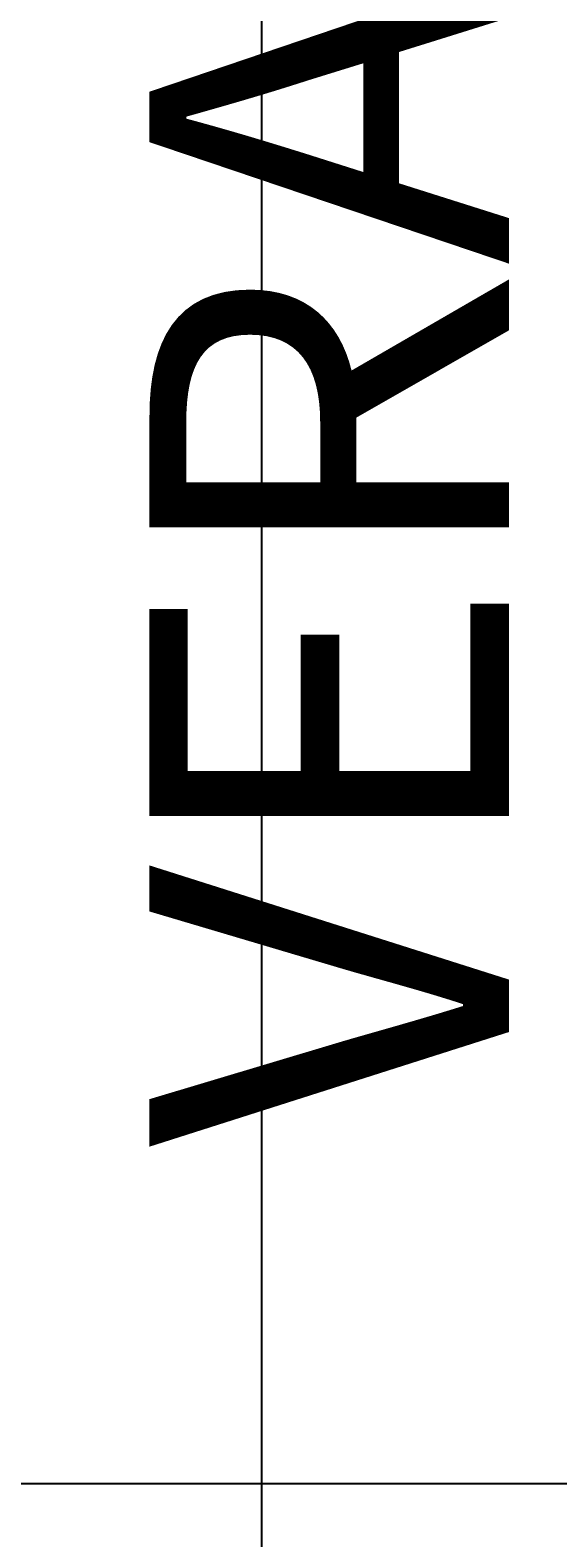
# Model space of a CAD drawing. Units: feet. Extents: x 1654 to 2985, y 1348 to 2230.
# Tile 11 of 53: x 2014 to 2027, y 1573 to 1608. Entities that reach past the tile are written whole.
import ezdxf

# ---------------------------------------------------------------- set-up
doc = ezdxf.new("R2010")
doc.units = ezdxf.units.FT
doc.layers.add('A-ANNO-DIMS', color=2, linetype='Continuous', lineweight=18)
doc.layers.add('A-AREA-IDEN', color=7, linetype='Continuous', lineweight=18)
doc.styles.get("Standard").update_dxf_attribs({"font": 'arial.ttf'})
doc.dimstyles.get("Standard").update_dxf_attribs({"dimtxt": 0.18, "dimasz": 0.18, "dimexe": 0.18, "dimexo": 0.0625, "dimgap": 0.09, "dimtad": 0, "dimtih": 1, "dimtoh": 1, "dimdec": 4, "dimzin": 0, "dimdsep": 46, "dimtxsty": 'Standard', "dimcen": 0.09, "dimadec": 0, "dimazin": 0, "dimtfac": 1, "dimtdec": 4, "dimtofl": 0, "dimtmove": 0, "dimatfit": 3, "dimfxl": 1, "dimtolj": 1, "dimtzin": 0, "dimarcsym": 0})

# ---------------------------------------------------------------- blocks, each defined once
blk = doc.blocks.new('*D90')
at = {"layer": 'A-ANNO-DIMS', "color": 0, "lineweight": -2, "transparency": 16777216}
for p, q in [((1852.155, 1641.187), (2242.272, 1641.187)), ((2242.092, 1641.007), (2242.092, 1607.903)), ((2242.092, 1574.435), (2242.092, 1607.539)), ((1852.155, 1574.255), (2242.272, 1574.255))]:
    blk.add_line(p, q, dxfattribs=at)
at = {"layer": 'A-ANNO-DIMS', "color": 0, "transparency": 16777216}
for points in [[(2242.062, 1641.007), (2242.122, 1641.007), (2242.092, 1641.187)], [(2242.062, 1574.435), (2242.122, 1574.435), (2242.092, 1574.255)]]:
    blk.add_solid(points, dxfattribs=at)
at = {"layer": 'Defpoints', "color": 0, "transparency": 16777216}
for p in [(1852.092, 1641.187), (2242.092, 1641.187), (1852.092, 1574.255)]:
    blk.add_point(p, dxfattribs=at)
at = {"layer": 'A-ANNO-DIMS', "color": 0, "transparency": 16777216, "insert": (2242.092, 1607.721), "char_height": 0.18, "attachment_point": 5}
blk.add_mtext('\\A1;66.93', dxfattribs=at)
blk = doc.blocks.new('*D102')
at = {"layer": 'A-ANNO-DIMS', "color": 0, "lineweight": -2, "transparency": 16777216}
for p, q in [((2008.092, 1742.192), (2008.092, 1534.075)), ((2019.757, 1742.192), (2019.757, 1534.075)), ((2008.272, 1534.255), (2013.47, 1534.255)), ((2019.577, 1534.255), (2014.379, 1534.255))]:
    blk.add_line(p, q, dxfattribs=at)
at = {"layer": 'A-ANNO-DIMS', "color": 0, "transparency": 16777216}
for points in [[(2008.272, 1534.285), (2008.272, 1534.225), (2008.092, 1534.255)], [(2019.577, 1534.285), (2019.577, 1534.225), (2019.757, 1534.255)]]:
    blk.add_solid(points, dxfattribs=at)
at = {"layer": 'Defpoints', "color": 0, "transparency": 16777216}
for p in [(2008.092, 1742.255), (2019.757, 1742.255), (2019.757, 1534.255)]:
    blk.add_point(p, dxfattribs=at)
at = {"layer": 'A-ANNO-DIMS', "color": 0, "transparency": 16777216, "insert": (2013.925, 1534.255), "char_height": 0.18, "attachment_point": 5}
blk.add_mtext('\\A1;11.664', dxfattribs=at)

msp = doc.modelspace()

# ---------------------------------------------------------------- texts
at = {"layer": 'A-AREA-IDEN'}
msp.add_text('VERANDAH', height=8.38114, rotation=90, dxfattribs=at).set_placement((2025.5306, 1582.1049))

# ---------------------------------------------------------------- dimensions: what is measured, and where the dimension line sits
at = {"layer": 'A-ANNO-DIMS'}
dim = msp.add_linear_dim(base=(2019.7567, 1534.2549), p1=(2008.0924, 1742.2549), p2=(2019.7567, 1742.2549), dimstyle='Standard', override={"dimdec": 3, "dimlfac": 1, "dimrnd": 0, "dimzin": 0, "dimdsep": 46, "dimlunit": 2}, dxfattribs=at)
dim.commit()
dim.dimension.update_dxf_attribs({"geometry": '*D102', "text_midpoint": (2013.9246, 1534.2549)})
dim = msp.add_linear_dim(base=(2242.0924, 1641.187), p1=(1852.0924, 1574.2549), p2=(1852.0924, 1641.187), angle=90, dimstyle='Standard', override={"dimdec": 2, "dimlfac": 1, "dimrnd": 0, "dimzin": 0, "dimdsep": 46, "dimlunit": 2}, dxfattribs=at)
dim.commit()
dim.dimension.update_dxf_attribs({"geometry": '*D90', "text_midpoint": (2242.0924, 1607.721)})

doc.saveas('drawing.dxf')
